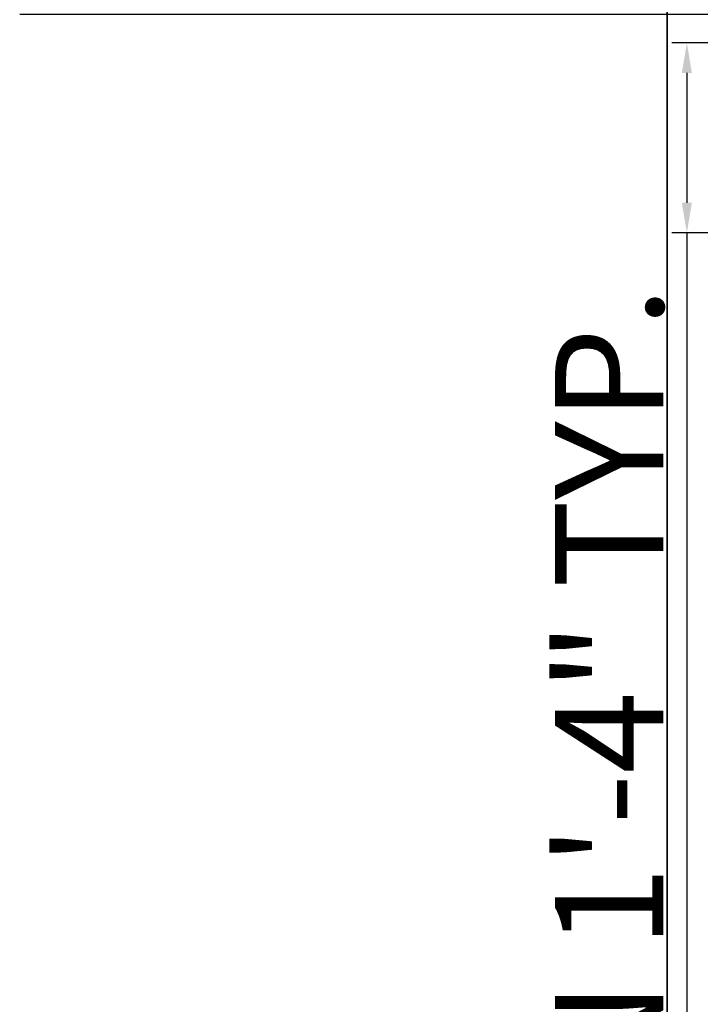
# Model space of a CAD drawing. Units: inches. Extents: x 3321 to 5237, y 11 to 1752.
# Tile 39 of 43: x 4886 to 4943, y 1598 to 1680. Entities that reach past the tile are written whole.
import ezdxf

# ---------------------------------------------------------------- set-up
doc = ezdxf.new("R2010")
doc.units = ezdxf.units.IN
doc.layers.add('A-ANNO-DIMS', color=2, linetype='Continuous', lineweight=18)
doc.layers.add('A-WALL', color=7, linetype='Continuous', lineweight=35)
doc.styles.get("Standard").update_dxf_attribs({"font": 'arial.ttf'})
doc.dimstyles.new('ISO-25', dxfattribs={"dimtxt": 9, "dimasz": 2.5, "dimexe": 1.25, "dimexo": 0.625, "dimtad": 1, "dimdec": 1, "dimlunit": 3, "dimtxsty": 'Standard', "dimcen": 2.5, "dimclrd": 4, "dimclre": 4, "dimclrt": 256, "dimadec": 0, "dimazin": 0, "dimtfac": 1, "dimtdec": 1, "dimtmove": 0, "dimatfit": 3, "dimfxl": 1, "dimarcsym": 0})

# ---------------------------------------------------------------- blocks, each defined once
blk = doc.blocks.new('*D201')
at = {"layer": 'A-ANNO-DIMS', "color": 4, "lineweight": -2, "transparency": 16777216}
for p, q in [((4943.459, 1678.339), (4940.467, 1678.339)), ((4941.717, 1675.839), (4941.717, 1665.058)), ((4943.459, 1662.558), (4940.467, 1662.558)), ((4941.717, 1662.558), (4941.717, 1563.124))]:
    blk.add_line(p, q, dxfattribs=at)
at = {"layer": 'A-ANNO-DIMS', "color": 4, "transparency": 16777216}
for points in [[(4941.3, 1675.839), (4942.134, 1675.839), (4941.717, 1678.339)], [(4941.3, 1665.058), (4942.134, 1665.058), (4941.717, 1662.558)]]:
    blk.add_solid(points, dxfattribs=at)
at = {"layer": 'Defpoints', "color": 0, "transparency": 16777216}
for p in [(4944.084, 1678.339), (4941.717, 1662.558), (4944.084, 1662.558)]:
    blk.add_point(p, dxfattribs=at)
at = {"layer": 'A-ANNO-DIMS', "transparency": 16777216, "insert": (4936.439, 1611.591), "char_height": 9, "attachment_point": 5, "rotation": 90}
blk.add_mtext('BASIN 1\'-4" TYP.', dxfattribs=at)
blk = doc.blocks.new('*D202')
at = {"layer": 'A-ANNO-DIMS', "color": 4, "lineweight": -2, "transparency": 16777216}
for p, q in [((4944.084, 1678.964), (4944.084, 1681.956)), ((4956.091, 1678.964), (4956.091, 1681.956)), ((4944.084, 1680.706), (4886.322, 1680.706)), ((4953.591, 1680.706), (4946.584, 1680.706))]:
    blk.add_line(p, q, dxfattribs=at)
at = {"layer": 'A-ANNO-DIMS', "color": 4, "transparency": 16777216}
for points in [[(4946.584, 1681.122), (4946.584, 1680.289), (4944.084, 1680.706)], [(4953.591, 1681.122), (4953.591, 1680.289), (4956.091, 1680.706)]]:
    blk.add_solid(points, dxfattribs=at)
at = {"layer": 'Defpoints', "color": 0, "transparency": 16777216}
for p in [(4944.084, 1680.706), (4944.084, 1678.339), (4956.091, 1678.339)]:
    blk.add_point(p, dxfattribs=at)
at = {"layer": 'A-ANNO-DIMS', "transparency": 16777216, "insert": (4913.953, 1685.926), "char_height": 9, "attachment_point": 5}
blk.add_mtext('1\'-0" TYP.', dxfattribs=at)

msp = doc.modelspace()

# ---------------------------------------------------------------- linework, layer by layer
at = {"layer": 'A-WALL'}
msp.add_line((4940.084, 1687.339), (4940.084, 1425.339), dxfattribs=at)

# ---------------------------------------------------------------- dimensions: what is measured, and where the dimension line sits
at = {"layer": 'A-ANNO-DIMS'}
for base, p1, p2, angle, text, picture, middle in [((4944.084, 1680.706), (4956.091, 1678.339), (4944.084, 1678.339), 180, '<> TYP.', '*D202', (4913.953, 1685.926)), ((4941.717, 1662.558), (4944.084, 1678.339), (4944.084, 1662.558), 270, 'BASIN <> TYP.', '*D201', (4936.439, 1611.591))]:
    dim = msp.add_linear_dim(base=base, p1=p1, p2=p2, angle=angle, text=text, dimstyle='ISO-25', override={"dimdec": 1, "dimlfac": 1, "dimrnd": 0, "dimzin": 1, "dimdsep": 46, "dimlunit": 4, "dimfrac": 2}, dxfattribs=at)
    dim.commit()
    dim.dimension.update_dxf_attribs({"geometry": picture, "text_midpoint": middle})

doc.saveas('drawing.dxf')
